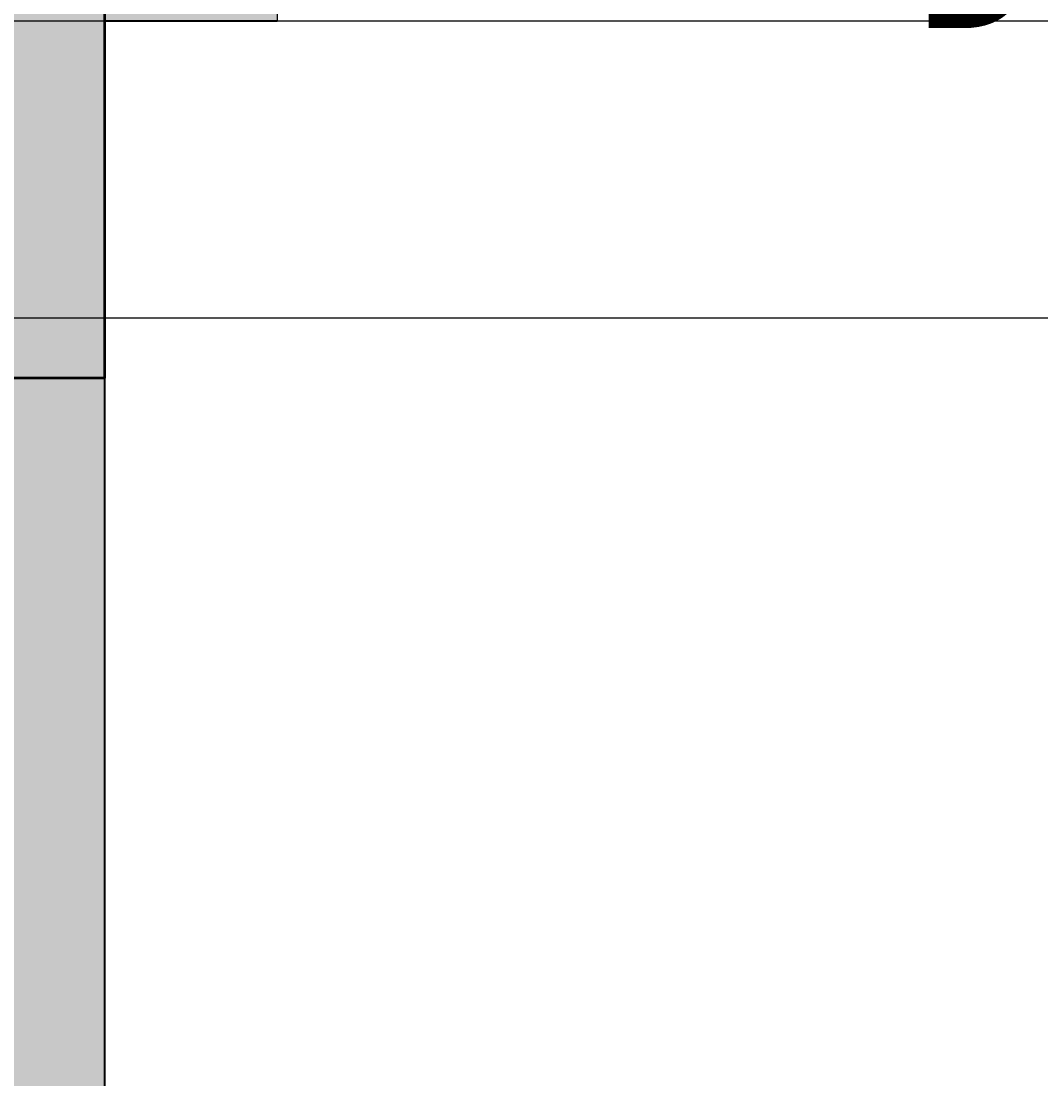
# Model space of a CAD drawing. Units: inches. Extents: x 1998 to 2588, y 1139 to 1977.
# Tile 97 of 134: x 2344 to 2371, y 1608 to 1637. Entities that reach past the tile are written whole.
import ezdxf

# ---------------------------------------------------------------- set-up
doc = ezdxf.new("R2010")
doc.units = ezdxf.units.IN
for name, color, linetype, lineweight in [('A-ANNO-DIMS', 2, 'Continuous', 18), ('A-COLS-PATT', 250, 'Continuous', 13), ('A-DOOR-IDEN', 7, 'Continuous', 18), ('A-WALL-PATT', 252, 'Continuous', 13), ('COLUMN', 10, 'Continuous', 50), ('DOOR', 52, 'Continuous', 25), ('WALL', 200, 'Continuous', 35)]:
    doc.layers.add(name, color=color, linetype=linetype, lineweight=lineweight)
doc.styles.get("Standard").update_dxf_attribs({"font": 'arial.ttf'})
doc.dimstyles.get("Standard").update_dxf_attribs({"dimtxt": 0.18, "dimasz": 0.18, "dimexe": 0.18, "dimexo": 0.0625, "dimgap": 0.09, "dimtad": 0, "dimtih": 1, "dimtoh": 1, "dimdec": 4, "dimzin": 0, "dimdsep": 46, "dimtxsty": 'Standard', "dimcen": 0.09, "dimadec": 0, "dimazin": 0, "dimtfac": 1, "dimtdec": 4, "dimtofl": 0, "dimtmove": 0, "dimatfit": 3, "dimfxl": 1, "dimtolj": 1, "dimtzin": 0, "dimarcsym": 0})

# ---------------------------------------------------------------- blocks, each defined once
blk = doc.blocks.new('*U2')
for p, q in [((0, 0), (0, -6)), ((40, 0), (40, -6))]:
    blk.add_line(p, q)
blk.add_lwpolyline([(0, 0), (0, 40), (1.75, 40), (1.75, 0)], close=True)
blk.add_arc((0, 0), 40, 0, 90)
blk = doc.blocks.new('*D30')
at = {"layer": 'A-ANNO-DIMS', "color": 0, "lineweight": -2, "transparency": 16777216}
for p, q in [((2407.91, 1636.732), (1997.843, 1636.732)), ((1998.023, 1636.552), (1998.023, 1615.913)), ((1998.023, 1594.912), (1998.023, 1615.552)), ((2407.91, 1594.732), (1997.843, 1594.732))]:
    blk.add_line(p, q, dxfattribs=at)
at = {"layer": 'A-ANNO-DIMS', "color": 0, "transparency": 16777216}
for points in [[(1997.993, 1636.552), (1998.053, 1636.552), (1998.023, 1636.732)], [(1997.993, 1594.912), (1998.053, 1594.912), (1998.023, 1594.732)]]:
    blk.add_solid(points, dxfattribs=at)
at = {"layer": 'Defpoints', "color": 0, "transparency": 16777216}
for p in [(1998.023, 1636.732), (2407.973, 1636.732), (2407.973, 1594.732)]:
    blk.add_point(p, dxfattribs=at)
at = {"layer": 'A-ANNO-DIMS', "color": 0, "transparency": 16777216, "insert": (1998.023, 1615.732), "char_height": 0.18, "attachment_point": 5}
blk.add_mtext('\\A1;42', dxfattribs=at)
blk = doc.blocks.new('*D39')
at = {"layer": 'A-ANNO-DIMS', "color": 0, "lineweight": -2, "transparency": 16777216}
for p, q in [((2115.035, 1628.742), (2588.309, 1628.742)), ((2588.129, 1628.562), (2588.129, 1612.685)), ((2588.129, 1596.444), (2588.129, 1612.321)), ((2115.035, 1596.264), (2588.309, 1596.264))]:
    blk.add_line(p, q, dxfattribs=at)
at = {"layer": 'A-ANNO-DIMS', "color": 0, "transparency": 16777216}
for points in [[(2588.099, 1628.562), (2588.159, 1628.562), (2588.129, 1628.742)], [(2588.099, 1596.444), (2588.159, 1596.444), (2588.129, 1596.264)]]:
    blk.add_solid(points, dxfattribs=at)
at = {"layer": 'Defpoints', "color": 0, "transparency": 16777216}
for p in [(2114.973, 1628.742), (2588.129, 1628.742), (2114.973, 1596.264)]:
    blk.add_point(p, dxfattribs=at)
at = {"layer": 'A-ANNO-DIMS', "color": 0, "transparency": 16777216, "insert": (2588.129, 1612.503), "char_height": 0.18, "attachment_point": 5}
blk.add_mtext('\\A1;32.48', dxfattribs=at)

msp = doc.modelspace()

# ---------------------------------------------------------------- hatches: boundary and pattern name
at = {"layer": 'A-COLS-PATT'}
h = msp.add_hatch(color=256, dxfattribs=at)
h.dxf.hatch_style = 1
h.paths.add_polyline_path([(2099.4125, 1888.7324), (2087.9729, 1888.7324), (2087.9729, 1868.3278), (2099.4125, 1868.3278)])
h.paths.add_polyline_path([(2234.4125, 1888.7324), (2222.9729, 1888.7324), (2222.9729, 1868.3278), (2234.4125, 1868.3278)])
h.paths.add_polyline_path([(2341.4729, 1886.637), (2330.0332, 1886.637), (2330.0332, 1866.2324), (2341.4729, 1866.2324)])
h.paths.add_polyline_path([(2507.8006, 1882.7324), (2487.396, 1882.7324), (2487.396, 1871.2927), (2507.8006, 1871.2927)])
h.paths.add_polyline_path([(2510.9729, 1766.672), (2490.5682, 1766.672), (2490.5682, 1755.2324), (2510.9729, 1755.2324)])
h.paths.add_polyline_path([(2345.9729, 1759.7324), (2334.5332, 1759.7324), (2334.5332, 1739.3278), (2345.9729, 1739.3278)])
h.paths.add_polyline_path([(2234.4125, 1774.3318), (2222.9729, 1774.3318), (2222.9729, 1753.9272), (2234.4125, 1753.9272)])
h.paths.add_polyline_path([(2099.4125, 1775.637), (2087.9729, 1775.637), (2087.9729, 1755.2324), (2099.4125, 1755.2324)])
h.paths.add_polyline_path([(2098.0956, 1593.7241), (2077.691, 1593.7241), (2077.691, 1582.2845), (2098.0956, 1582.2845)])
h.paths.add_polyline_path([(2227.4729, 1604.637), (2216.0332, 1604.637), (2216.0332, 1584.2324), (2227.4729, 1584.2324)])
h.paths.add_polyline_path([(2345.9729, 1647.5211), (2334.5332, 1647.5211), (2334.5332, 1627.1165), (2345.9729, 1627.1165)])
h.paths.add_polyline_path([(2522.3775, 1641.2324), (2501.9729, 1641.2324), (2501.9729, 1629.7927), (2522.3775, 1629.7927)])
h.paths.add_polyline_path([(2522.3775, 1480.7324), (2501.9729, 1480.7324), (2501.9729, 1469.2927), (2522.3775, 1469.2927)])
h.paths.add_polyline_path([(2345.9729, 1488.5616), (2334.5332, 1488.5616), (2334.5332, 1468.1569), (2345.9729, 1468.1569)])
h.paths.add_polyline_path([(2234.4125, 1486.137), (2227.4729, 1486.137), (2227.4729, 1465.7324), (2234.4125, 1465.7324)])
h.paths.add_polyline_path([(2227.4729, 1486.137), (2222.9729, 1486.137), (2222.9729, 1465.7324), (2227.4729, 1465.7324)])
h.paths.add_polyline_path([(2108.3775, 1470.2324), (2087.9729, 1470.2324), (2087.9729, 1458.7927), (2108.3775, 1458.7927)])
h.paths.add_polyline_path([(2096.9729, 1365.5012), (2087.9729, 1365.5012), (2087.9729, 1345.0966), (2096.9729, 1345.0966)])
h.paths.add_polyline_path([(2087.9729, 1365.5012), (2085.5332, 1365.5012), (2085.5332, 1345.0966), (2087.9729, 1345.0966)])
h.paths.add_polyline_path([(2234.4125, 1285.137), (2222.9729, 1285.137), (2222.9729, 1264.7324), (2234.4125, 1264.7324)])
h.paths.add_polyline_path([(2345.9729, 1285.137), (2334.5332, 1285.137), (2334.5332, 1264.7324), (2345.9729, 1264.7324)])
h.paths.add_polyline_path([(2503.1458, 1240.172), (2482.7412, 1240.172), (2482.7412, 1228.7324), (2503.1458, 1228.7324)])
h.paths.add_polyline_path([(2510.9729, 1369.172), (2490.5682, 1369.172), (2490.5682, 1357.7324), (2510.9729, 1357.7324)])
at = {"layer": 'A-WALL-PATT'}
h = msp.add_hatch(color=256, dxfattribs=at)
h.dxf.hatch_style = 1
h.paths.add_polyline_path([(2222.9729, 1888.7324), (2099.4125, 1888.7324), (2099.4125, 1879.7324), (2222.9729, 1879.7324)])
h.paths.add_polyline_path([(2096.9729, 1868.3278), (2087.9729, 1868.3278), (2087.9729, 1775.637), (2096.9729, 1775.637)])
h.paths.add_polyline_path([(2227.4729, 1868.3278), (2222.9729, 1868.3278), (2222.9729, 1774.3318), (2227.4729, 1774.3318)])
h.paths.add_polyline_path([(2188.3019, 1759.7324), (2138.6074, 1759.7324), (2099.4125, 1759.7324), (2099.4125, 1755.2324), (2176.9729, 1755.2324), (2188.3019, 1755.2324)])
h.paths.add_polyline_path([(2087.9729, 1759.7324), (2059.4729, 1759.7324), (2059.4729, 1702.7324), (2087.9729, 1702.7324), (2087.9729, 1707.2324), (2063.9729, 1707.2324), (2063.9729, 1755.2324), (2087.9729, 1755.2324)])
h.paths.add_polyline_path([(2096.9729, 1755.2324), (2087.9729, 1755.2324), (2087.9729, 1707.2324), (2096.9729, 1707.2324)])
h.paths.add_polyline_path([(2187.0461, 1707.2324), (2105.9729, 1707.2324), (2096.9729, 1707.2324), (2087.9729, 1707.2324), (2087.9729, 1702.7324), (2105.9729, 1702.7324), (2114.9729, 1702.7324), (2187.0461, 1702.7324)])
h.paths.add_polyline_path([(2181.4729, 1719.2028), (2176.9729, 1719.2028), (2176.9729, 1707.2324), (2181.4729, 1707.2324)])
h.paths.add_polyline_path([(2216.0332, 1588.7324), (2114.9729, 1588.7324), (2105.9729, 1588.7324), (2105.9729, 1584.2324), (2216.0332, 1584.2324)])
h.paths.add_polyline_path([(2077.691, 1588.7324), (2061.4729, 1588.7324), (2061.4729, 1584.2324), (2077.691, 1584.2324)])
h.paths.add_polyline_path([(2105.9729, 1588.7324), (2098.0956, 1588.7324), (2098.0956, 1584.2324), (2105.9729, 1584.2324)])
h.paths.add_polyline_path([(2114.9729, 1596.2642), (2110.1012, 1596.2642), (2105.9729, 1596.2642), (2105.9729, 1588.7324), (2114.9729, 1588.7324)])
h.paths.add_polyline_path([(2114.9729, 1584.2324), (2105.9729, 1584.2324), (2105.9729, 1580.249), (2110.1012, 1580.249), (2114.9729, 1580.249)])
h.paths.add_polyline_path([(2114.9729, 1547.7716), (2110.1012, 1547.7716, -0.0318759), (2105.9729, 1548.035), (2105.9729, 1470.2324), (2108.3775, 1470.2324), (2108.3775, 1465.7324), (2186.2943, 1465.7324), (2186.2943, 1470.2324), (2114.9729, 1470.2324)])
h.paths.add_polyline_path([(2227.4729, 1584.2324), (2222.9729, 1584.2324), (2222.9729, 1486.137), (2227.4729, 1486.137)])
h.paths.add_polyline_path([(2295.4138, 1593.2324), (2227.4729, 1593.2324), (2227.4729, 1588.7324), (2295.4138, 1588.7324), (2295.4138, 1591.8729)])
h.paths.add_polyline_path([(2345.9729, 1627.1165), (2341.4729, 1627.1165), (2341.4729, 1593.2324), (2337.2869, 1593.2324), (2337.2869, 1591.8729), (2337.2869, 1588.7324), (2345.9729, 1588.7324)])
h.paths.add_polyline_path([(2291.9729, 1588.7324), (2287.4729, 1588.7324), (2287.4729, 1522.7324), (2291.9729, 1522.7324)])
h.paths.add_polyline_path([(2291.9729, 1522.7324), (2287.4729, 1522.7324), (2227.4729, 1522.7324), (2227.4729, 1518.2324), (2291.9729, 1518.2324)])
h.paths.add_polyline_path([(2295.7347, 1519.5919), (2295.7347, 1522.7324), (2291.9729, 1522.7324), (2291.9729, 1518.2324), (2295.7347, 1518.2324)])
h.paths.add_polyline_path([(2345.9729, 1522.7324), (2337.6078, 1522.7324), (2337.6078, 1519.5919), (2337.6078, 1518.2324), (2341.4729, 1518.2324), (2341.4729, 1488.5616), (2345.9729, 1488.5616)])
h.paths.add_polyline_path([(2345.9729, 1468.1569), (2341.4729, 1468.1569), (2341.4729, 1374.2324), (2227.4729, 1374.2324), (2227.4729, 1369.7324), (2345.9729, 1369.7324)])
h.paths.add_polyline_path([(2345.9729, 1369.7324), (2341.4729, 1369.7324), (2341.4729, 1362.2324), (2345.9729, 1362.2324)])
h.paths.add_polyline_path([(2345.9729, 1317.7324), (2345.9729, 1322.2324), (2341.4729, 1322.2324), (2341.4729, 1285.137), (2345.9729, 1285.137)], flags=17)
h.paths.add_polyline_path([(2356.2096, 1322.2324), (2345.9729, 1322.2324), (2345.9729, 1317.7324), (2356.2096, 1317.7324), (2356.2096, 1319.3088)], flags=17)
h.paths.add_polyline_path([(2393.9729, 1322.2324), (2375.6999, 1322.2324), (2375.6999, 1319.3088, -0.0202458), (2375.636, 1317.7324), (2393.9729, 1317.7324)], flags=17)
h.paths.add_polyline_path([(2398.4729, 1322.2324), (2393.9729, 1322.2324), (2393.9729, 1317.7324), (2393.9729, 1237.7324), (2345.9729, 1237.7324), (2345.9729, 1264.7324), (2341.4729, 1264.7324), (2341.4729, 1228.7324), (2393.9729, 1228.7324), (2482.7412, 1228.7324), (2482.7412, 1237.7324), (2398.4729, 1237.7324), (2398.4729, 1297.1029)])
h.paths.add_polyline_path([(2398.4729, 1362.2324), (2393.9729, 1362.2324), (2393.9729, 1357.7324), (2398.4729, 1357.7324)])
h.paths.add_polyline_path([(2345.9729, 1329.7549), (2341.4729, 1329.7549), (2341.4729, 1322.2324), (2345.9729, 1322.2324)])
h = msp.add_hatch(color=256, dxfattribs=at)
h.dxf.hatch_style = 1
h.paths.add_polyline_path([(2527.4729, 1362.2324), (2510.9729, 1362.2324), (2510.9729, 1357.7324), (2518.4729, 1357.7324), (2518.4729, 1237.7324), (2503.1458, 1237.7324), (2503.1458, 1228.7324), (2527.4729, 1228.7324)])
h.paths.add_polyline_path([(2490.5682, 1362.2324), (2398.4729, 1362.2324), (2398.4729, 1357.7324), (2490.5682, 1357.7324)])
h.paths.add_polyline_path([(2224.9729, 1264.7324), (2222.9729, 1264.7324), (2222.9729, 1232.4125), (2341.4729, 1232.4125), (2341.4729, 1234.4125), (2224.9729, 1234.4125)])
h.paths.add_polyline_path([(2334.5332, 1273.7324), (2264.7638, 1273.7324), (2264.7638, 1269.5611, -0.043659), (2264.3413, 1264.7324), (2334.5332, 1264.7324)])
h.paths.add_polyline_path([(2236.9551, 1273.7324), (2234.4125, 1273.7324), (2234.4125, 1264.7324), (2236.9551, 1264.7324), (2236.9551, 1269.5611)])
h.paths.add_polyline_path([(2222.9729, 1293.2324), (2096.9729, 1293.2324), (2096.9729, 1345.0966), (2087.9729, 1345.0966), (2087.9729, 1284.2324), (2222.9729, 1284.2324), (2222.9729, 1285.137)])
h.paths.add_polyline_path([(2096.9729, 1458.7927), (2087.9729, 1458.7927), (2087.9729, 1417.7324), (2087.9729, 1413.2324), (2096.9729, 1413.2324), (2096.9729, 1417.7324)])
h.paths.add_polyline_path([(2096.9729, 1413.2324), (2087.9729, 1413.2324), (2087.9729, 1365.5012), (2096.9729, 1365.5012), (2096.9729, 1369.3358)])
h.paths.add_polyline_path([(2186.2943, 1417.7324), (2138.6074, 1417.7324), (2096.9729, 1417.7324), (2096.9729, 1413.2324), (2138.6074, 1413.2324), (2186.2943, 1413.2324)])
h.paths.add_polyline_path([(2181.4729, 1465.7324), (2176.9729, 1465.7324), (2176.9729, 1451.6434), (2181.4729, 1451.6434)])
h.paths.add_polyline_path([(2181.4729, 1422.1664), (2176.9729, 1422.1664), (2176.9729, 1417.7324), (2181.4729, 1417.7324)])
h.paths.add_polyline_path([(2063.9729, 1465.7324), (2087.9729, 1465.7324), (2087.9729, 1470.2324), (2059.4729, 1470.2324), (2059.4729, 1413.2324), (2087.9729, 1413.2324), (2087.9729, 1417.7324), (2063.9729, 1417.7324)])
h.paths.add_polyline_path([(2181.4729, 1755.2324), (2176.9729, 1755.2324), (2176.9729, 1748.6798), (2177.0513, 1748.6798), (2181.4729, 1748.6798)])
h.paths.add_polyline_path([(2227.4729, 1707.2324), (2220.4647, 1707.2324), (2220.4647, 1702.7324), (2222.9729, 1702.7324), (2222.9729, 1604.637), (2227.4729, 1604.637)])
h.paths.add_polyline_path([(2114.9729, 1702.7324), (2105.9729, 1702.7324), (2105.9729, 1628.4781, -0.0318759), (2110.1012, 1628.7416), (2114.9729, 1628.7416)])
h.paths.add_polyline_path([(2345.9729, 1739.3278), (2341.4729, 1739.3278), (2341.4729, 1647.5211), (2345.9729, 1647.5211)])
h.paths.add_polyline_path([(2350.6273, 1641.2324), (2345.9729, 1641.2324), (2345.9729, 1636.7324), (2350.6273, 1636.7324), (2350.6273, 1639.8729)])
h.paths.add_polyline_path([(2501.9729, 1641.2324), (2407.9729, 1641.2324), (2392.5005, 1641.2324), (2392.5005, 1639.8729), (2392.5005, 1636.7324), (2501.9729, 1636.7324)])
h.paths.add_polyline_path([(2510.9729, 1755.2324), (2501.9729, 1755.2324), (2501.9729, 1641.2324), (2510.9729, 1641.2324)])
h.paths.add_polyline_path([(2549.1786, 1641.2324), (2522.3775, 1641.2324), (2522.3775, 1636.7324), (2540.1786, 1636.7324), (2540.1786, 1480.7324), (2522.3775, 1480.7324), (2522.3775, 1476.2324), (2549.1786, 1476.2324)])
h.paths.add_polyline_path([(2498.1786, 1594.7324), (2407.9729, 1594.7324), (2407.9729, 1585.7324), (2416.9729, 1585.7324), (2489.1786, 1585.7324), (2489.1786, 1531.7324), (2416.9729, 1531.7324), (2407.9729, 1531.7324), (2407.9729, 1522.7324), (2498.1786, 1522.7324)])
h.paths.add_polyline_path([(2351.6437, 1480.7324), (2345.9729, 1480.7324), (2345.9729, 1476.2324), (2351.6437, 1476.2324), (2351.6437, 1477.5919)])
h.paths.add_polyline_path([(2501.9729, 1480.7324), (2498.1786, 1480.7324), (2407.9729, 1480.7324), (2393.5168, 1480.7324), (2393.5168, 1477.5919), (2393.5168, 1476.2324), (2501.9729, 1476.2324)])

# ---------------------------------------------------------------- linework, layer by layer
at = {"layer": 'COLUMN'}
msp.add_lwpolyline([(2334.5332, 1647.5211), (2345.9729, 1647.5211), (2345.9729, 1627.1165), (2334.5332, 1627.1165)], close=True, dxfattribs=at)
at = {"layer": 'WALL'}
for p, q in [((2345.9729, 1755.2324), (2345.9729, 1588.7324)), ((2345.9729, 1636.7324), (2345.9729, 1588.7324)), ((2350.6273, 1636.7324), (2345.9729, 1636.7324))]:
    msp.add_line(p, q, dxfattribs=at)

# ---------------------------------------------------------------- block references
at = {"layer": 'DOOR', "xscale": 0.5234138920659225, "yscale": 0.5234138920659225, "zscale": 0.5234138920659225}
msp.add_blockref('*U2', (2350.6273, 1639.8729), dxfattribs=at)

# ---------------------------------------------------------------- texts
at = {"layer": 'A-DOOR-IDEN', "insert": (2367.677, 1640.2432), "char_height": 3.6988, "attachment_point": 1}
msp.add_mtext_dynamic_manual_height_columns('D', width=110.572713, gutter_width=18.4938, heights=[0], dxfattribs=at)

# ---------------------------------------------------------------- dimensions: what is measured, and where the dimension line sits
at = {"layer": 'A-ANNO-DIMS'}
for base, p1, p2, override, picture, middle in [((1998.0229, 1636.7324), (2407.9729, 1594.7324), (2407.9729, 1636.7324), {"dimdec": 0, "dimlfac": 1, "dimrnd": 0, "dimzin": 0, "dimdsep": 46, "dimlunit": 2}, '*D30', (1998.0229, 1615.7324)), ((2588.1286, 1628.7416), (2114.9729, 1596.2642), (2114.9729, 1628.7416), {"dimdec": 2, "dimlfac": 1, "dimrnd": 0, "dimzin": 0, "dimdsep": 46, "dimlunit": 2}, '*D39', (2588.1286, 1612.5029))]:
    dim = msp.add_linear_dim(base=base, p1=p1, p2=p2, angle=90, dimstyle='Standard', override=override, dxfattribs=at)
    dim.commit()
    dim.dimension.update_dxf_attribs({"geometry": picture, "text_midpoint": middle})

doc.saveas('drawing.dxf')
